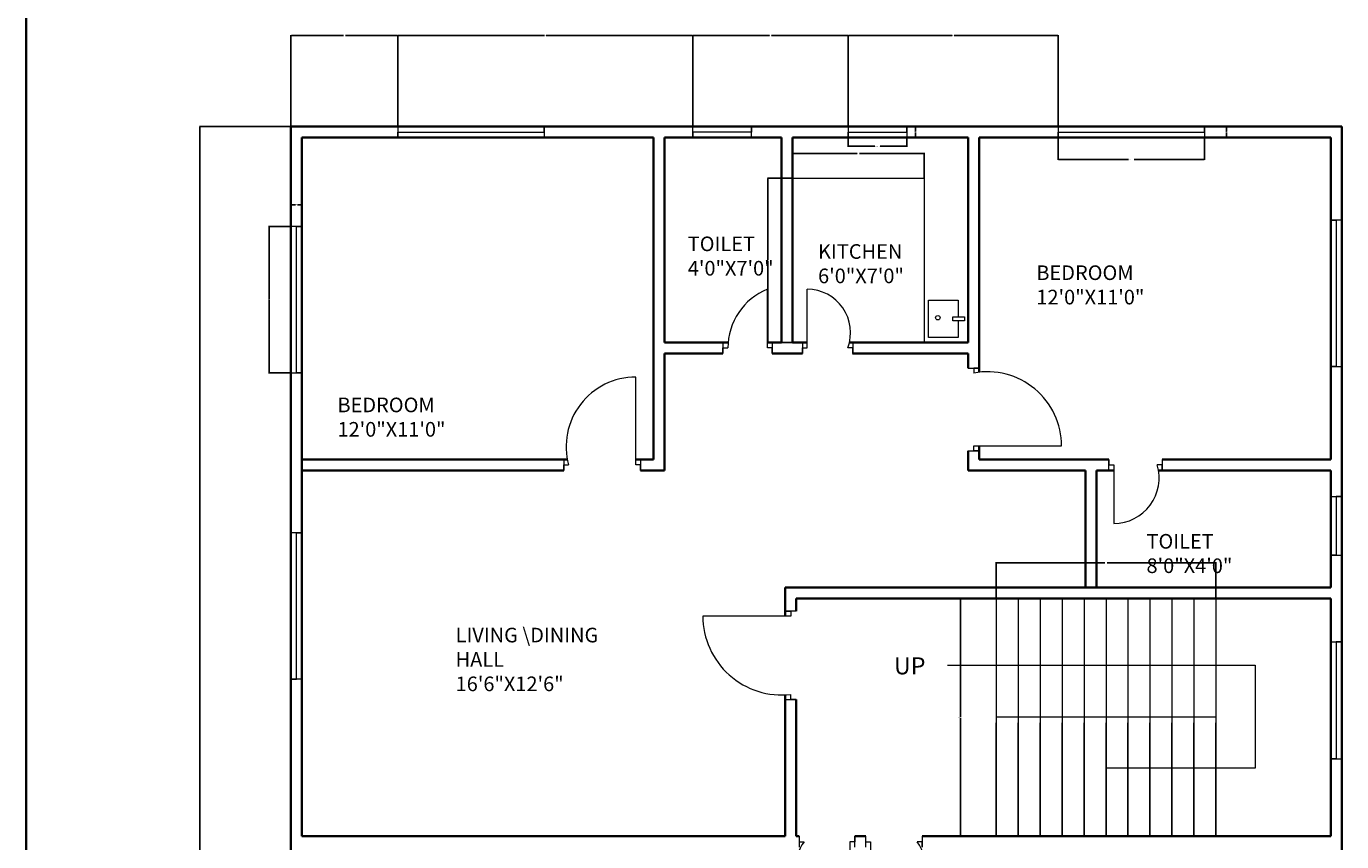
# Model space of a CAD drawing. Units: inches. Extents: x 992 to 2287, y 1476 to 2866.
# Tile 2 of 9: x 992 to 1531, y 1987 to 2321. Entities that reach past the tile are written whole.
import ezdxf

# ---------------------------------------------------------------- set-up
doc = ezdxf.new("R2010")
doc.units = ezdxf.units.IN
for name, color, linetype, lineweight in [('A-ANNO-DIMS', 2, 'Continuous', 18), ('A-ANNO-SYMB', 2, 'Continuous', 18), ('A-ANNO-TTLB', 7, 'Continuous', 35), ('A-AREA-IDEN', 7, 'Continuous', 18), ('A-DOOR', 3, 'Continuous', 18), ('A-FLOR-CASE', 9, 'Continuous', 18), ('A-FLOR-FIXT', 8, 'Continuous', 18), ('A-FLOR-STRS', 7, 'Continuous', 18), ('A-GLAZ', 4, 'Continuous', 18), ('A-WALL', 7, 'Continuous', 35)]:
    doc.layers.add(name, color=color, linetype=linetype, lineweight=lineweight)
doc.styles.get("Standard").update_dxf_attribs({"font": 'arial.ttf'})
doc.dimstyles.get("Standard").update_dxf_attribs({"dimtxt": 0.18, "dimasz": 0.18, "dimexe": 0.18, "dimexo": 0.0625, "dimgap": 0.09, "dimtad": 0, "dimtih": 1, "dimtoh": 1, "dimdec": 4, "dimzin": 0, "dimdsep": 46, "dimtxsty": 'Standard', "dimcen": 0.09, "dimadec": 0, "dimazin": 0, "dimtfac": 1, "dimtdec": 4, "dimtofl": 0, "dimtmove": 0, "dimatfit": 3, "dimfxl": 1, "dimtolj": 1, "dimtzin": 0, "dimarcsym": 0})

# ---------------------------------------------------------------- blocks, each defined once
blk = doc.blocks.new('DOOR-SINGLE-36IN-01')
for p, q in [((36, 34.15), (0, 34.15)), ((38.25, 36.15), (33.75, 36.15)), ((33.75, 36.15), (36, 36.15)), ((36, 36.15), (36, 34.15)), ((33.75, 0), (38.25, 0)), ((36, 0), (36, 2)), ((38.25, 0), (36, 0))]:
    blk.add_line(p, q)
blk.add_arc((32.36, 34.15), 32.36, 180, 276.4675)
blk = doc.blocks.new('DOOR-SINGLE-36IN-02')
for p, q in [((0, 33.92), (4.5, 33.92)), ((4.5, 33.92), (2.25, 33.92)), ((2.25, 33.92), (2.25, 31.92)), ((0, 0), (4.5, 0)), ((2.25, 0), (2.25, 2)), ((2.25, 2), (38.25, 2)), ((4.5, 0), (2.25, 0))]:
    blk.add_line(p, q)
blk.add_arc((7.81, 2), 30.44, 0, 100.535)
blk = doc.blocks.new('DOOR-SINGLE-24IN-03')
for p, q in [((0, 21.75), (0, 26.25)), ((0, 26.25), (0, 24)), ((0, 24), (0, 24)), ((0, 24), (2, 24)), ((2, 24), (2, 0)), ((21.76, 24), (19.76, 24)), ((21.76, 26.25), (21.76, 21.75)), ((21.76, 21.75), (21.76, 24))]:
    blk.add_line(p, q)
blk.add_arc((2, 18.57), 18.57, 270, 16.9925)
blk = doc.blocks.new('DOOR-SINGLE-24IN-04')
for p, q in [((18.2, 2.25), (18.2, 26.25)), ((0, 4.5), (0, 0)), ((0, 0), (0, 2.25)), ((0, 2.25), (2, 2.25)), ((20.2, 2.25), (18.2, 2.25)), ((20.2, 4.5), (20.2, 0)), ((20.2, 0), (20.2, 2.25))]:
    blk.add_line(p, q)
blk.add_arc((27.88, 2.25), 25.88, 111.9643, 180)
blk = doc.blocks.new('DOOR-SINGLE-24IN-05')
for p, q in [((2, 2.25), (2, 26.25)), ((0, 4.5), (0, 0)), ((0, 0), (0, 2.25)), ((0, 2.25), (2, 2.25)), ((20.6, 2.25), (18.6, 2.25)), ((20.6, 4.5), (20.6, 0)), ((20.6, 0), (20.6, 2.25))]:
    blk.add_line(p, q)
blk.add_arc((2, 8.51), 17.74, 339.3303, 90)
blk = doc.blocks.new('DOOR-SINGLE-36IN-06')
for p, q in [((29.52, 2.25), (29.52, 38.25)), ((0, 4.5), (0, 0)), ((0, 0), (0, 2.25)), ((0, 2.25), (2, 2.25)), ((31.52, 2.25), (29.52, 2.25)), ((31.52, 4.5), (31.52, 0)), ((31.52, 0), (31.52, 2.25))]:
    blk.add_line(p, q)
blk.add_arc((29.52, 9.74), 28.51, 90, 195.2187)
blk = doc.blocks.new('DOOR-SINGLE-36IN-07')
for p, q in [((2.12, 38.25), (2.12, 33.75)), ((24.9, 33.75), (24.9, 38.25)), ((24.9, 38.25), (24.9, 36)), ((2.12, 36), (4.12, 36)), ((24.9, 36), (22.9, 36)), ((22.9, 36), (22.9, 0))]:
    blk.add_line(p, q)
blk.add_arc((22.9, 22.9), 22.9, 145.0915, 270)
blk = doc.blocks.new('DOOR-SINGLE-36IN-08')
for p, q in [((0, 33.75), (0, 38.25)), ((23.12, 38.25), (23.12, 33.75)), ((0, 36), (2, 36)), ((2, 36), (2, 0)), ((23.12, 36), (21.12, 36)), ((23.12, 33.75), (23.12, 36))]:
    blk.add_line(p, q)
blk.add_arc((2, 23.08), 23.08, 270, 34.0417)
blk = doc.blocks.new('WINDOW-24IN-A')
for p, q in [((0, 24), (4.5, 24)), ((4.5, 24), (2.25, 24)), ((2.25, 24), (2.25, 0)), ((2.25, 0), (0, 0)), ((0, 0), (4.5, 0))]:
    blk.add_line(p, q)
blk = doc.blocks.new('WINDOW-60IN-A')
for p, q in [((4.5, 60), (0, 60)), ((0, 60), (2.25, 60)), ((2.25, 60), (2.25, 0)), ((2.25, 0), (0, 0)), ((0, 0), (4.5, 0))]:
    blk.add_line(p, q)
blk = doc.blocks.new('WINDOW-60IN-B')
for p, q in [((0, 4.5), (0, 0)), ((0, 0), (0, 2.25)), ((0, 2.25), (60, 2.25)), ((60, 2.25), (60, 4.5)), ((60, 4.5), (60, 0))]:
    blk.add_line(p, q)
blk = doc.blocks.new('WINDOW-24IN-B')
for p, q in [((0, 4.5), (0, 4.5)), ((0, 4.5), (0, 0)), ((0, 0), (0, 2.25)), ((0, 2.25), (24, 2.25)), ((24, 2.25), (24, 4.5)), ((24, 4.5), (24, 0))]:
    blk.add_line(p, q)
blk = doc.blocks.new('STAIR-RETURN-PLAN')
for p, q in [((0, 97.5), (0, 0)), ((9, 97.5), (9, 0)), ((18, 97.5), (18, 0)), ((27, 97.5), (27, 0)), ((36, 97.5), (36, 0)), ((45, 97.5), (45, 0)), ((54, 97.5), (54, 0)), ((63, 97.5), (63, 0)), ((72, 97.5), (72, 0)), ((81, 97.5), (81, 0)), ((90, 97.5), (90, 0)), ((90, 48.75), (0, 48.75)), ((0, 0), (0, 46.5)), ((9, 0), (9, 46.5)), ((18, 0), (18, 46.5)), ((27, 0), (27, 46.5)), ((36, 0), (36, 46.5)), ((45, 0), (45, 46.5)), ((54, 0), (54, 46.5)), ((63, 0), (63, 46.5)), ((72, 0), (72, 46.5)), ((81, 0), (81, 46.5)), ((90, 0), (90, 46.5))]:
    blk.add_line(p, q)
blk = doc.blocks.new('COUNTER-L-NORTH')
for p, q in [((0, 67.36), (53.88, 67.36)), ((53.88, 67.36), (53.88, 0))]:
    blk.add_line(p, q)
blk = doc.blocks.new('*D37')
at = {"layer": 'A-ANNO-DIMS', "color": 0, "lineweight": -2, "transparency": 16777216}
for p, q in [((1415.12, 2275.48), (1415.12, 2266.36)), ((1475.12, 2275.48), (1475.12, 2266.36)), ((1415.3, 2266.54), (1444, 2266.54)), ((1474.94, 2266.54), (1446.24, 2266.54))]:
    blk.add_line(p, q, dxfattribs=at)
at = {"layer": 'A-ANNO-DIMS', "color": 0, "transparency": 16777216}
for points in [[(1415.3, 2266.57), (1415.3, 2266.51), (1415.12, 2266.54)], [(1474.94, 2266.57), (1474.94, 2266.51), (1475.12, 2266.54)]]:
    blk.add_solid(points, dxfattribs=at)
at = {"layer": 'Defpoints', "color": 0, "transparency": 16777216}
for p in [(1415.12, 2275.54), (1475.12, 2275.54), (1475.12, 2266.54)]:
    blk.add_point(p, dxfattribs=at)
at = {"layer": 'A-ANNO-DIMS', "color": 0, "transparency": 16777216, "insert": (1445.12, 2266.54), "char_height": 0.18, "attachment_point": 5}
blk.add_mtext('\\A1;WINDOW 60 TYP.', dxfattribs=at)
blk = doc.blocks.new('*D38')
at = {"layer": 'A-ANNO-DIMS', "color": 0, "lineweight": -2, "transparency": 16777216}
for p, q in [((1475.18, 2280.04), (1484.3, 2280.04)), ((1484.12, 2279.86), (1484.12, 2277.97)), ((1475.18, 2275.54), (1484.3, 2275.54)), ((1484.12, 2275.72), (1484.12, 2277.61))]:
    blk.add_line(p, q, dxfattribs=at)
at = {"layer": 'A-ANNO-DIMS', "color": 0, "transparency": 16777216}
for points in [[(1484.09, 2279.86), (1484.15, 2279.86), (1484.12, 2280.04)], [(1484.09, 2275.72), (1484.15, 2275.72), (1484.12, 2275.54)]]:
    blk.add_solid(points, dxfattribs=at)
at = {"layer": 'Defpoints', "color": 0, "transparency": 16777216}
for p in [(1475.12, 2280.04), (1484.12, 2280.04), (1475.12, 2275.54)]:
    blk.add_point(p, dxfattribs=at)
at = {"layer": 'A-ANNO-DIMS', "color": 0, "transparency": 16777216, "insert": (1484.12, 2277.79), "char_height": 0.18, "attachment_point": 5}
blk.add_mtext('\\A1;5 TYP.', dxfattribs=at)
blk = doc.blocks.new('*D41')
at = {"layer": 'A-ANNO-DIMS', "color": 0, "lineweight": -2, "transparency": 16777216}
for p, q in [((1100.73, 2239), (1091.61, 2239)), ((1091.79, 2238.82), (1091.79, 2209.18)), ((1091.79, 2179.18), (1091.79, 2208.82)), ((1100.73, 2179), (1091.61, 2179))]:
    blk.add_line(p, q, dxfattribs=at)
at = {"layer": 'A-ANNO-DIMS', "color": 0, "transparency": 16777216}
for points in [[(1091.76, 2238.82), (1091.82, 2238.82), (1091.79, 2239)], [(1091.76, 2179.18), (1091.82, 2179.18), (1091.79, 2179)]]:
    blk.add_solid(points, dxfattribs=at)
at = {"layer": 'Defpoints', "color": 0, "transparency": 16777216}
for p in [(1100.79, 2239), (1091.79, 2179), (1100.79, 2179)]:
    blk.add_point(p, dxfattribs=at)
at = {"layer": 'A-ANNO-DIMS', "color": 0, "transparency": 16777216, "insert": (1091.79, 2209), "char_height": 0.18, "attachment_point": 5}
blk.add_mtext('\\A1;WINDOW 60 TYP.', dxfattribs=at)
blk = doc.blocks.new('*D42')
at = {"layer": 'A-ANNO-DIMS', "color": 0, "lineweight": -2, "transparency": 16777216}
for p, q in [((1100.79, 2239.06), (1100.79, 2248.18)), ((1100.97, 2248), (1102.59, 2248)), ((1105.11, 2248), (1103.5, 2248)), ((1105.29, 2239.06), (1105.29, 2248.18))]:
    blk.add_line(p, q, dxfattribs=at)
at = {"layer": 'A-ANNO-DIMS', "color": 0, "transparency": 16777216}
for points in [[(1100.97, 2248.03), (1100.97, 2247.97), (1100.79, 2248)], [(1105.11, 2248.03), (1105.11, 2247.97), (1105.29, 2248)]]:
    blk.add_solid(points, dxfattribs=at)
at = {"layer": 'Defpoints', "color": 0, "transparency": 16777216}
for p in [(1100.79, 2248), (1100.79, 2239), (1105.29, 2239)]:
    blk.add_point(p, dxfattribs=at)
at = {"layer": 'A-ANNO-DIMS', "color": 0, "transparency": 16777216, "insert": (1103.04, 2248), "char_height": 0.18, "attachment_point": 5}
blk.add_mtext('\\A1;5 TYP.', dxfattribs=at)
blk = doc.blocks.new('*D47')
at = {"layer": 'A-ANNO-DIMS', "color": 0, "lineweight": -2, "transparency": 16777216}
for p, q in [((1329.08, 2275.48), (1329.08, 2271.76)), ((1353.08, 2275.48), (1353.08, 2271.76)), ((1329.26, 2271.94), (1339.96, 2271.94)), ((1352.9, 2271.94), (1342.2, 2271.94))]:
    blk.add_line(p, q, dxfattribs=at)
at = {"layer": 'A-ANNO-DIMS', "color": 0, "transparency": 16777216}
for points in [[(1329.26, 2271.97), (1329.26, 2271.91), (1329.08, 2271.94)], [(1352.9, 2271.97), (1352.9, 2271.91), (1353.08, 2271.94)]]:
    blk.add_solid(points, dxfattribs=at)
at = {"layer": 'Defpoints', "color": 0, "transparency": 16777216}
for p in [(1329.08, 2275.54), (1353.08, 2275.54), (1353.08, 2271.94)]:
    blk.add_point(p, dxfattribs=at)
at = {"layer": 'A-ANNO-DIMS', "color": 0, "transparency": 16777216, "insert": (1341.08, 2271.94), "char_height": 0.18, "attachment_point": 5}
blk.add_mtext('\\A1;WINDOW 24 TYP.', dxfattribs=at)
blk = doc.blocks.new('*D48')
at = {"layer": 'A-ANNO-DIMS', "color": 0, "lineweight": -2, "transparency": 16777216}
for p, q in [((1353.15, 2280.04), (1356.86, 2280.04)), ((1356.68, 2279.86), (1356.68, 2277.97)), ((1353.15, 2275.54), (1356.86, 2275.54)), ((1356.68, 2275.72), (1356.68, 2277.61))]:
    blk.add_line(p, q, dxfattribs=at)
at = {"layer": 'A-ANNO-DIMS', "color": 0, "transparency": 16777216}
for points in [[(1356.65, 2279.86), (1356.71, 2279.86), (1356.68, 2280.04)], [(1356.65, 2275.72), (1356.71, 2275.72), (1356.68, 2275.54)]]:
    blk.add_solid(points, dxfattribs=at)
at = {"layer": 'Defpoints', "color": 0, "transparency": 16777216}
for p in [(1353.08, 2280.04), (1356.68, 2280.04), (1353.08, 2275.54)]:
    blk.add_point(p, dxfattribs=at)
at = {"layer": 'A-ANNO-DIMS', "color": 0, "transparency": 16777216, "insert": (1356.68, 2277.79), "char_height": 0.18, "attachment_point": 5}
blk.add_mtext('\\A1;5 TYP.', dxfattribs=at)
blk = doc.blocks.new('*D85')
at = {"layer": 'A-ANNO-DIMS', "color": 0, "lineweight": -2, "transparency": 16777216}
for p, q in [((1389.66, 2086.54), (1374.92, 2086.54)), ((1375.1, 2086.36), (1375.1, 2037.98)), ((1375.1, 1989.22), (1375.1, 2037.61)), ((1389.66, 1989.04), (1374.92, 1989.04))]:
    blk.add_line(p, q, dxfattribs=at)
at = {"layer": 'A-ANNO-DIMS', "color": 0, "transparency": 16777216}
for points in [[(1375.07, 2086.36), (1375.13, 2086.36), (1375.1, 2086.54)], [(1375.07, 1989.22), (1375.13, 1989.22), (1375.1, 1989.04)]]:
    blk.add_solid(points, dxfattribs=at)
at = {"layer": 'Defpoints', "color": 0, "transparency": 16777216}
for p in [(1375.1, 2086.54), (1389.73, 2086.54), (1389.73, 1989.04)]:
    blk.add_point(p, dxfattribs=at)
at = {"layer": 'A-ANNO-DIMS', "color": 0, "transparency": 16777216, "insert": (1375.1, 2037.79), "char_height": 0.18, "attachment_point": 5}
blk.add_mtext('\\A1;STAIR 98 TYP.', dxfattribs=at)
blk = doc.blocks.new('*D86')
at = {"layer": 'A-ANNO-DIMS', "color": 0, "lineweight": -2, "transparency": 16777216}
for p, q in [((1389.73, 2086.61), (1389.73, 2101.35)), ((1389.91, 2101.17), (1434.2, 2101.17)), ((1479.55, 2101.17), (1435.25, 2101.17)), ((1479.73, 2086.61), (1479.73, 2101.35))]:
    blk.add_line(p, q, dxfattribs=at)
at = {"layer": 'A-ANNO-DIMS', "color": 0, "transparency": 16777216}
for points in [[(1389.91, 2101.2), (1389.91, 2101.14), (1389.73, 2101.17)], [(1479.55, 2101.2), (1479.55, 2101.14), (1479.73, 2101.17)]]:
    blk.add_solid(points, dxfattribs=at)
at = {"layer": 'Defpoints', "color": 0, "transparency": 16777216}
for p in [(1479.73, 2101.17), (1389.73, 2086.54), (1479.73, 2086.54)]:
    blk.add_point(p, dxfattribs=at)
at = {"layer": 'A-ANNO-DIMS', "color": 0, "transparency": 16777216, "insert": (1434.73, 2101.17), "char_height": 0.18, "attachment_point": 5}
blk.add_mtext('\\A1;90 TYP.', dxfattribs=at)
blk = doc.blocks.new('*D91')
at = {"layer": 'A-ANNO-DIMS', "color": 0, "lineweight": -2, "transparency": 16777216}
for p, q in [((1306.23, 2258.9), (1296.01, 2258.9)), ((1296.19, 2258.72), (1296.19, 2225.41)), ((1296.19, 2191.72), (1296.19, 2225.04)), ((1306.23, 2191.54), (1296.01, 2191.54))]:
    blk.add_line(p, q, dxfattribs=at)
at = {"layer": 'A-ANNO-DIMS', "color": 0, "transparency": 16777216}
for points in [[(1296.16, 2258.72), (1296.22, 2258.72), (1296.19, 2258.9)], [(1296.16, 2191.72), (1296.22, 2191.72), (1296.19, 2191.54)]]:
    blk.add_solid(points, dxfattribs=at)
at = {"layer": 'Defpoints', "color": 0, "transparency": 16777216}
for p in [(1296.19, 2258.9), (1306.29, 2258.9), (1306.29, 2191.54)]:
    blk.add_point(p, dxfattribs=at)
at = {"layer": 'A-ANNO-DIMS', "color": 0, "transparency": 16777216, "insert": (1296.19, 2225.22), "char_height": 0.18, "attachment_point": 5}
blk.add_mtext('\\A1;COUNTER 67 TYP.', dxfattribs=at)
blk = doc.blocks.new('*D92')
at = {"layer": 'A-ANNO-DIMS', "color": 0, "lineweight": -2, "transparency": 16777216}
for p, q in [((1306.29, 2258.97), (1306.29, 2269.19)), ((1306.47, 2269.01), (1332.71, 2269.01)), ((1360, 2269.01), (1333.76, 2269.01)), ((1360.18, 2258.97), (1360.18, 2269.19))]:
    blk.add_line(p, q, dxfattribs=at)
at = {"layer": 'A-ANNO-DIMS', "color": 0, "transparency": 16777216}
for points in [[(1306.47, 2269.04), (1306.47, 2268.98), (1306.29, 2269.01)], [(1360, 2269.04), (1360, 2268.98), (1360.18, 2269.01)]]:
    blk.add_solid(points, dxfattribs=at)
at = {"layer": 'Defpoints', "color": 0, "transparency": 16777216}
for p in [(1360.18, 2269.01), (1306.29, 2258.9), (1360.18, 2258.9)]:
    blk.add_point(p, dxfattribs=at)
at = {"layer": 'A-ANNO-DIMS', "color": 0, "transparency": 16777216, "insert": (1333.24, 2269.01), "char_height": 0.18, "attachment_point": 5}
blk.add_mtext('\\A1;54 TYP.', dxfattribs=at)
blk = doc.blocks.new('*D110')
at = {"layer": 'A-ANNO-DIMS', "color": 0, "lineweight": -2, "transparency": 16777216}
for p, q in [((1100.73, 2280.04), (1063.31, 2280.04)), ((1063.49, 2279.86), (1063.49, 1955.47)), ((1063.49, 1630.72), (1063.49, 1955.11)), ((1100.73, 1630.54), (1063.31, 1630.54))]:
    blk.add_line(p, q, dxfattribs=at)
at = {"layer": 'A-ANNO-DIMS', "color": 0, "transparency": 16777216}
for points in [[(1063.46, 2279.86), (1063.52, 2279.86), (1063.49, 2280.04)], [(1063.46, 1630.72), (1063.52, 1630.72), (1063.49, 1630.54)]]:
    blk.add_solid(points, dxfattribs=at)
at = {"layer": 'Defpoints', "color": 0, "transparency": 16777216}
for p in [(1063.49, 2280.04), (1100.79, 2280.04), (1100.79, 1630.54)]:
    blk.add_point(p, dxfattribs=at)
at = {"layer": 'A-ANNO-DIMS', "color": 0, "transparency": 16777216, "insert": (1063.49, 1955.29), "char_height": 0.18, "attachment_point": 5}
blk.add_mtext('\\A1;649.5', dxfattribs=at)
blk = doc.blocks.new('*D113')
at = {"layer": 'A-ANNO-DIMS', "color": 0, "lineweight": -2, "transparency": 16777216}
for p, q in [((1100.79, 2280.11), (1100.79, 2317.52)), ((1144.55, 2280.11), (1144.55, 2317.52)), ((1100.97, 2317.34), (1122.28, 2317.34)), ((1144.37, 2317.34), (1123.07, 2317.34))]:
    blk.add_line(p, q, dxfattribs=at)
at = {"layer": 'A-ANNO-DIMS', "color": 0, "transparency": 16777216}
for points in [[(1100.97, 2317.37), (1100.97, 2317.31), (1100.79, 2317.34)], [(1144.37, 2317.37), (1144.37, 2317.31), (1144.55, 2317.34)]]:
    blk.add_solid(points, dxfattribs=at)
at = {"layer": 'Defpoints', "color": 0, "transparency": 16777216}
for p in [(1144.55, 2317.34), (1100.79, 2280.04), (1144.55, 2280.04)]:
    blk.add_point(p, dxfattribs=at)
at = {"layer": 'A-ANNO-DIMS', "color": 0, "transparency": 16777216, "insert": (1122.67, 2317.34), "char_height": 0.18, "attachment_point": 5}
blk.add_mtext('\\A1;43.76', dxfattribs=at)
blk = doc.blocks.new('*D114')
at = {"layer": 'A-ANNO-DIMS', "color": 0, "lineweight": -2, "transparency": 16777216}
for p, q in [((1144.55, 2280.11), (1144.55, 2317.52)), ((1265.45, 2280.11), (1265.45, 2317.52)), ((1144.73, 2317.34), (1204.62, 2317.34)), ((1265.27, 2317.34), (1205.39, 2317.34))]:
    blk.add_line(p, q, dxfattribs=at)
at = {"layer": 'A-ANNO-DIMS', "color": 0, "transparency": 16777216}
for points in [[(1144.73, 2317.37), (1144.73, 2317.31), (1144.55, 2317.34)], [(1265.27, 2317.37), (1265.27, 2317.31), (1265.45, 2317.34)]]:
    blk.add_solid(points, dxfattribs=at)
at = {"layer": 'Defpoints', "color": 0, "transparency": 16777216}
for p in [(1265.45, 2317.34), (1144.55, 2280.04), (1265.45, 2280.04)]:
    blk.add_point(p, dxfattribs=at)
at = {"layer": 'A-ANNO-DIMS', "color": 0, "transparency": 16777216, "insert": (1205, 2317.34), "char_height": 0.18, "attachment_point": 5}
blk.add_mtext('\\A1;120.9', dxfattribs=at)
blk = doc.blocks.new('*D115')
at = {"layer": 'A-ANNO-DIMS', "color": 0, "lineweight": -2, "transparency": 16777216}
for p, q in [((1265.45, 2280.11), (1265.45, 2317.52)), ((1329.08, 2280.11), (1329.08, 2317.52)), ((1265.63, 2317.34), (1296.87, 2317.34)), ((1328.9, 2317.34), (1297.66, 2317.34))]:
    blk.add_line(p, q, dxfattribs=at)
at = {"layer": 'A-ANNO-DIMS', "color": 0, "transparency": 16777216}
for points in [[(1265.63, 2317.37), (1265.63, 2317.31), (1265.45, 2317.34)], [(1328.9, 2317.37), (1328.9, 2317.31), (1329.08, 2317.34)]]:
    blk.add_solid(points, dxfattribs=at)
at = {"layer": 'Defpoints', "color": 0, "transparency": 16777216}
for p in [(1329.08, 2317.34), (1265.45, 2280.04), (1329.08, 2280.04)]:
    blk.add_point(p, dxfattribs=at)
at = {"layer": 'A-ANNO-DIMS', "color": 0, "transparency": 16777216, "insert": (1297.27, 2317.34), "char_height": 0.18, "attachment_point": 5}
blk.add_mtext('\\A1;63.64', dxfattribs=at)
blk = doc.blocks.new('*D116')
at = {"layer": 'A-ANNO-DIMS', "color": 0, "lineweight": -2, "transparency": 16777216}
for p, q in [((1329.08, 2280.11), (1329.08, 2317.52)), ((1415.12, 2280.11), (1415.12, 2317.52)), ((1329.26, 2317.34), (1371.71, 2317.34)), ((1414.94, 2317.34), (1372.5, 2317.34))]:
    blk.add_line(p, q, dxfattribs=at)
at = {"layer": 'A-ANNO-DIMS', "color": 0, "transparency": 16777216}
for points in [[(1329.26, 2317.37), (1329.26, 2317.31), (1329.08, 2317.34)], [(1414.94, 2317.37), (1414.94, 2317.31), (1415.12, 2317.34)]]:
    blk.add_solid(points, dxfattribs=at)
at = {"layer": 'Defpoints', "color": 0, "transparency": 16777216}
for p in [(1415.12, 2317.34), (1329.08, 2280.04), (1415.12, 2280.04)]:
    blk.add_point(p, dxfattribs=at)
at = {"layer": 'A-ANNO-DIMS', "color": 0, "transparency": 16777216, "insert": (1372.1, 2317.34), "char_height": 0.18, "attachment_point": 5}
blk.add_mtext('\\A1;86.04', dxfattribs=at)

msp = doc.modelspace()

# ---------------------------------------------------------------- linework, layer by layer
at = {"layer": 'A-ANNO-SYMB'}
for p, q in [((1369.7251, 2059.2025), (1495.8569, 2059.2025)), ((1495.8569, 2059.2025), (1495.8569, 2016.9738)), ((1495.8569, 2016.9738), (1434.7267, 2016.9738))]:
    msp.add_line(p, q, dxfattribs=at)
at = {"layer": 'A-ANNO-TTLB'}
msp.add_lwpolyline([(992.3484, 2866.1952), (2287.217, 2866.1952), (2287.217, 1476.4066), (992.3484, 1476.4066)], close=True, dxfattribs=at)
at = {"layer": 'A-FLOR-FIXT'}
msp.add_lwpolyline([(1374.2133, 2200.3438), (1374.2133, 2193.5395), (1362.0485, 2193.5395), (1362.0485, 2208.8821), (1374.2133, 2208.8821), (1374.2133, 2202.0778)], dxfattribs=at)
msp.add_lwpolyline([(1372.0175, 2202.0778), (1376.8044, 2202.0778), (1376.8044, 2200.3438), (1372.0175, 2200.3438)], close=True, dxfattribs=at)
msp.add_circle((1365.8253, 2201.6388), 0.8999, dxfattribs=at)
at = {"layer": 'A-GLAZ'}
for p, q in [((1526.7936, 2068.7863), (1531.2936, 2068.7863)), ((1531.2936, 2068.7863), (1529.0436, 2068.7863)), ((1529.0436, 2068.7863), (1529.0436, 2020.7863)), ((1529.0436, 2020.7863), (1526.7936, 2020.7863)), ((1526.7936, 2020.7863), (1531.2936, 2020.7863))]:
    msp.add_line(p, q, dxfattribs=at)
at = {"layer": 'A-WALL'}
for p, q in [((1100.7936, 2280.0428), (1531.2936, 2280.0428)), ((1100.7936, 2280.0428), (1531.2936, 2280.0428)), ((1100.7936, 2280.0428), (1100.7936, 1677.0428)), ((1531.2936, 2280.0428), (1531.2936, 1677.0428)), ((1105.2936, 2275.5428), (1249.2936, 2275.5428)), ((1105.2936, 2275.5428), (1105.2936, 1989.0428)), ((1249.2936, 2275.5428), (1249.2936, 2143.5428)), ((1253.7936, 2275.5428), (1253.7936, 2191.5428)), ((1253.7936, 2275.5428), (1301.7936, 2275.5428)), ((1301.7936, 2275.5428), (1301.7936, 2191.5428)), ((1306.2936, 2275.5428), (1306.2936, 2191.5428)), ((1306.2936, 2275.5428), (1378.2936, 2275.5428)), ((1378.2936, 2275.5428), (1378.2936, 2191.5428)), ((1382.7936, 2275.5428), (1382.7936, 2179.3035)), ((1382.7936, 2275.5428), (1526.7936, 2275.5428)), ((1526.7936, 2275.5428), (1526.7936, 2143.5428)), ((1253.7936, 2191.5428), (1279.8915, 2191.5428)), ((1295.9926, 2191.5428), (1301.7936, 2191.5428)), ((1306.2936, 2191.5428), (1312.3308, 2191.5428)), ((1329.6099, 2191.5428), (1378.2936, 2191.5428)), ((1253.7936, 2187.0428), (1277.7936, 2187.0428)), ((1253.7936, 2187.0428), (1253.7936, 2139.0428)), ((1297.9926, 2187.0428), (1301.7936, 2187.0428)), ((1301.7936, 2187.0428), (1310.3308, 2187.0428)), ((1330.9276, 2187.0428), (1378.2936, 2187.0428)), ((1378.2936, 2187.0428), (1378.2936, 2180.9715)), ((1378.2936, 2147.0492), (1378.2936, 2139.0428)), ((1382.7936, 2149.0492), (1382.7936, 2143.5428)), ((1105.2936, 2143.5428), (1214.0111, 2143.5428)), ((1242.0411, 2143.5428), (1249.2936, 2143.5428)), ((1382.7936, 2143.5428), (1435.9175, 2143.5428)), ((1457.679, 2143.5428), (1526.7936, 2143.5428)), ((1105.2936, 2139.0428), (1212.5264, 2139.0428)), ((1244.0411, 2139.0428), (1253.7936, 2139.0428)), ((1382.7936, 2139.0428), (1378.2936, 2139.0428)), ((1382.7936, 2139.0428), (1426.2936, 2139.0428)), ((1426.2936, 2091.0428), (1426.2936, 2139.0428)), ((1430.7936, 2139.0428), (1430.7936, 2091.0428)), ((1430.7936, 2139.0428), (1437.9175, 2139.0428)), ((1437.9175, 2139.0428), (1430.7936, 2139.0428)), ((1526.7936, 2139.0428), (1456.2159, 2139.0428)), ((1456.2159, 2139.0428), (1526.7936, 2139.0428)), ((1526.7936, 2139.0428), (1526.7936, 2091.0428)), ((1303.2936, 2091.0428), (1526.7936, 2091.0428)), ((1303.2936, 2091.0428), (1303.2936, 2079.3118)), ((1307.7936, 2086.5428), (1526.7936, 2086.5428)), ((1307.7936, 2086.5428), (1307.7936, 2081.3118)), ((1430.7936, 2091.0428), (1426.2936, 2091.0428)), ((1526.7936, 2086.5428), (1526.7936, 1989.0428)), ((1303.2936, 2046.9864), (1303.2936, 1989.0428)), ((1307.7936, 2045.1622), (1307.7936, 1989.0428)), ((1105.2936, 1989.0428), (1303.2936, 1989.0428)), ((1307.7936, 1989.0428), (1309.0166, 1989.0428)), ((1331.7936, 1989.0428), (1336.2936, 1989.0428)), ((1359.4183, 1989.0428), (1526.7936, 1989.0428)), ((1531.2936, 1989.0428), (1531.2936, 1984.5428))]:
    msp.add_line(p, q, dxfattribs=at)

# ---------------------------------------------------------------- block references
at = {"layer": 'A-DOOR'}
for name, p in [('DOOR-SINGLE-24IN-04', (1277.794, 2187.043)), ('DOOR-SINGLE-24IN-05', (1310.331, 2187.043)), ('DOOR-SINGLE-36IN-02', (1378.294, 2147.049)), ('DOOR-SINGLE-36IN-06', (1212.526, 2139.043)), ('DOOR-SINGLE-24IN-03', (1435.917, 2117.293)), ('DOOR-SINGLE-36IN-01', (1269.544, 2045.162)), ('DOOR-SINGLE-36IN-07', (1306.897, 1950.793)), ('DOOR-SINGLE-36IN-08', (1336.294, 1950.793))]:
    msp.add_blockref(name, p, dxfattribs=at)
at = {"layer": 'A-FLOR-CASE'}
msp.add_blockref('COUNTER-L-NORTH', (1306.294, 2191.543), dxfattribs=at)
at = {"layer": 'A-FLOR-STRS'}
msp.add_blockref('STAIR-RETURN-PLAN', (1389.727, 1989.043), dxfattribs=at)
at = {"layer": 'A-GLAZ'}
for name, p in [('WINDOW-60IN-B', (1144.5536, 2275.543)), ('WINDOW-24IN-B', (1329.083, 2275.543)), ('WINDOW-60IN-B', (1415.122, 2275.543)), ('WINDOW-60IN-A', (1526.794, 2181.633)), ('WINDOW-24IN-A', (1526.794, 2104.303))]:
    msp.add_blockref(name, p, dxfattribs=at)
at = {"layer": 'A-GLAZ', "extrusion": (0, 0, -1), "zscale": -1, "rotation": 90}
for name, p in [('WINDOW-24IN-A', (-1265.4485, 2275.5432)), ('WINDOW-60IN-B', (-1100.7938, 2053.4168))]:
    msp.add_blockref(name, p, dxfattribs=at)
at = {"layer": 'A-GLAZ', "rotation": 180}
msp.add_blockref('WINDOW-60IN-A', (1105.2931, 2239.0001), dxfattribs=at)

# ---------------------------------------------------------------- texts
at = {"layer": 'A-ANNO-SYMB', "insert": (1347.8433, 2062.4009), "char_height": 7, "attachment_point": 1}
msp.add_mtext_dynamic_manual_height_columns('UP', width=15.522402, gutter_width=12.5, heights=[0], dxfattribs=at)
at = {"layer": 'A-AREA-IDEN', "char_height": 6, "attachment_point": 1}
for s, width, insert in [('TOILET\\P4\'0"X7\'0"', 52.098958, (1263.3665, 2234.9385)), ('KITCHEN\\P6\'0"X7\'0"', 58.950922, (1316.7516, 2231.7976)), ('BEDROOM\\P12\'0"X11\'0"', 93.45208, (1406.1892, 2223.1034)), ('BEDROOM\\P12\'0"X11\'0"', 88.803548, (1119.8386, 2168.8868)), ('TOILET\\P8\'0"X4\'0"', 84.958006, (1451.3254, 2112.9633)), ('LIVING \\\\DINING HALL\\P16\'6"X12\'6"', 77.886548, (1168.2562, 2074.5274))]:
    msp.add_mtext_dynamic_manual_height_columns(s, width=width, gutter_width=12.5, heights=[0], dxfattribs=dict(at, insert=insert))

# ---------------------------------------------------------------- dimensions: what is measured, and where the dimension line sits
at = {"layer": 'A-ANNO-DIMS'}
for base, p1, p2, override, picture, middle in [((1144.5539, 2317.3428), (1100.7936, 2280.0428), (1144.5539, 2280.0428), {"dimdec": 2, "dimlfac": 1, "dimrnd": 0, "dimzin": 0, "dimdsep": 46, "dimlunit": 2}, '*D113', (1122.6737, 2317.3428)), ((1265.4482, 2317.3428), (1144.5539, 2280.0428), (1265.4482, 2280.0428), {"dimdec": 1, "dimlfac": 1, "dimrnd": 0, "dimzin": 0, "dimdsep": 46, "dimlunit": 2}, '*D114', (1205.001, 2317.3428)), ((1329.08323, 2317.34279), (1265.44818, 2280.04279), (1329.08323, 2280.04279), {"dimdec": 2, "dimlfac": 1, "dimrnd": 0, "dimzin": 0, "dimdsep": 46, "dimlunit": 2}, '*D115', (1297.26571, 2317.34279)), ((1415.1222, 2317.3428), (1329.0832, 2280.0428), (1415.1222, 2280.0428), {"dimdec": 2, "dimlfac": 1, "dimrnd": 0, "dimzin": 0, "dimdsep": 46, "dimlunit": 2}, '*D116', (1372.1027, 2317.3428))]:
    dim = msp.add_linear_dim(base=base, p1=p1, p2=p2, dimstyle='Standard', override=override, dxfattribs=at)
    dim.commit()
    dim.dimension.update_dxf_attribs({"geometry": picture, "text_midpoint": middle})
dim = msp.add_linear_dim(base=(1063.4936, 2280.0428), p1=(1100.7936, 1630.5428), p2=(1100.7936, 2280.0428), angle=90, dimstyle='Standard', override={"dimdec": 1, "dimlfac": 1, "dimrnd": 0, "dimzin": 0, "dimdsep": 46, "dimlunit": 2}, dxfattribs=at)
dim.commit()
dim.dimension.update_dxf_attribs({"geometry": '*D110', "text_midpoint": (1063.4936, 1955.2928)})
for base, p1, p2, angle, text, picture, middle in [((1356.683231298, 2280.042787875), (1353.083231298, 2275.542787875), (1353.083231298, 2280.042787875), 90, '<> TYP.', '*D48', (1356.683231298, 2277.792787875)), ((1484.1222458426, 2280.042787875), (1475.1222458426, 2275.542787875), (1475.1222458426, 2280.042787875), 90, '<> TYP.', '*D38', (1484.1222458426, 2277.792787875)), ((1296.1894, 2258.9038), (1306.2936, 2191.5428), (1306.2936, 2258.9038), 90, 'COUNTER <> TYP.', '*D91', (1296.1894, 2225.2233)), ((1100.7935507769, 2248.0001094305), (1105.2935507769, 2239.0001094305), (1100.7935507769, 2239.0001094305), 180, '<> TYP.', '*D42', (1103.0435507769, 2248.0001094305)), ((1091.7936, 2179.0001), (1100.7936, 2239.0001), (1100.7936, 2179.0001), 270, 'WINDOW <> TYP.', '*D41', (1091.7936, 2209.0001)), ((1375.1017155153, 2086.542787875), (1389.7267155153, 1989.042787875), (1389.7267155153, 2086.542787875), 90, 'STAIR <> TYP.', '*D85', (1375.1017155153, 2037.792787875))]:
    dim = msp.add_linear_dim(base=base, p1=p1, p2=p2, angle=angle, text=text, dimstyle='Standard', override={"dimdec": 0, "dimlfac": 1, "dimrnd": 0, "dimzin": 0, "dimdsep": 46, "dimlunit": 2}, dxfattribs=at)
    dim.commit()
    dim.dimension.update_dxf_attribs({"geometry": picture, "text_midpoint": middle})
for base, p1, p2, text, picture, middle in [((1353.0832, 2271.9428), (1329.0832, 2275.5428), (1353.0832, 2275.5428), 'WINDOW <> TYP.', '*D47', (1341.0832, 2271.9428)), ((1475.1222, 2266.5428), (1415.1222, 2275.5428), (1475.1222, 2275.5428), 'WINDOW <> TYP.', '*D37', (1445.1222, 2266.5428)), ((1360.1788, 2269.008), (1306.2936, 2258.9038), (1360.1788, 2258.9038), '<> TYP.', '*D92', (1333.2362, 2269.008)), ((1479.7267, 2101.1678), (1389.7267, 2086.5428), (1479.7267, 2086.5428), '<> TYP.', '*D86', (1434.7267, 2101.1678))]:
    dim = msp.add_linear_dim(base=base, p1=p1, p2=p2, text=text, dimstyle='Standard', override={"dimdec": 0, "dimlfac": 1, "dimrnd": 0, "dimzin": 0, "dimdsep": 46, "dimlunit": 2}, dxfattribs=at)
    dim.commit()
    dim.dimension.update_dxf_attribs({"geometry": picture, "text_midpoint": middle})

doc.saveas('drawing.dxf')
